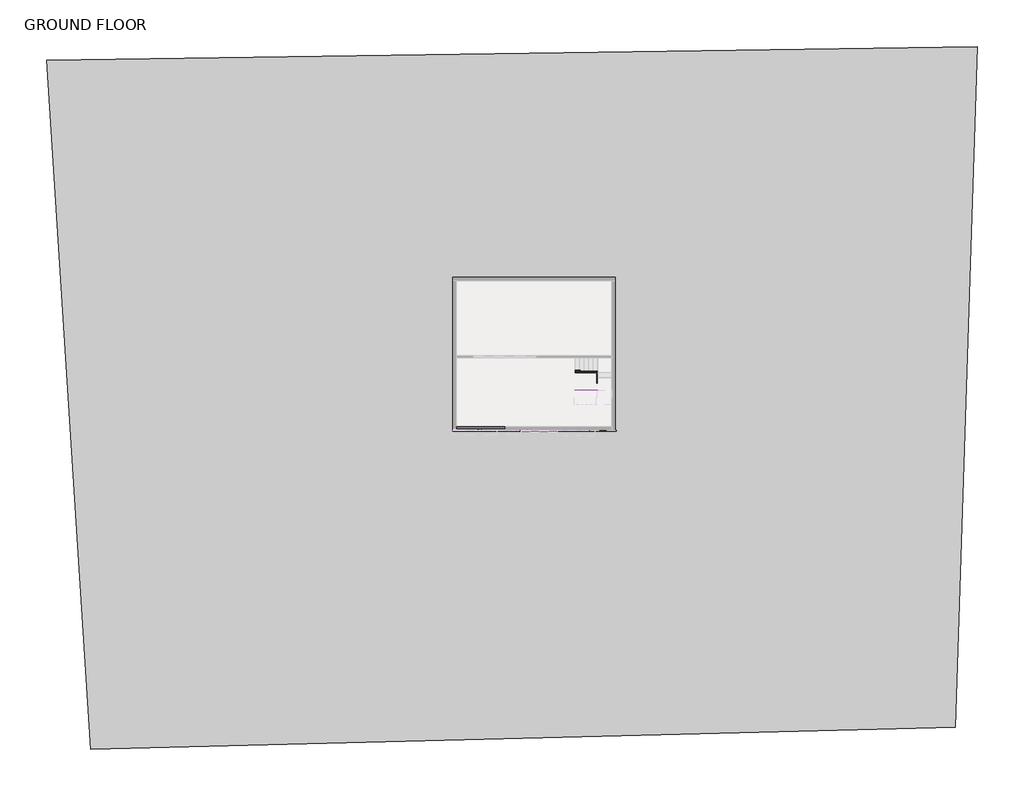
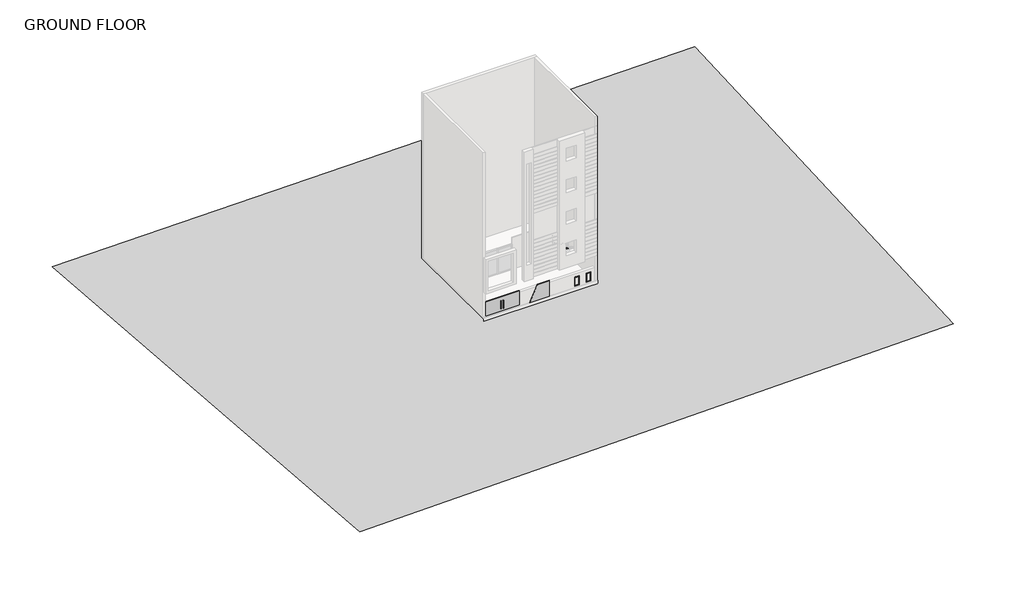
# One storey, part 3 of 3: 4 members, 3 proxies, 1 railing.
"""IFC4 building model written with IfcOpenShell, lengths in millimetres."""

from ifc_helpers import new_model, si_unit, frame, origin, place, context, project, spatial, polyline, circle_curve, ellipse_curve, outline, extrude, triangles, transform, mapped, element, save
from ifc_brep_helpers import plane_surface, cylinder_surface, advanced_brep
from components import generic_models_1_generic_models_1_bb1f4732, generic_models_2_generic_models_2_568ed07e

model = new_model("IFC4")

# Units and contexts
model_context = context("Model", 3, world=origin())
ifc_project = project(units=[si_unit("LENGTHUNIT", "METRE", prefix="MILLI")], contexts=[model_context])

# Site, building, storey
site = spatial("IfcSite", under=ifc_project)
building = spatial("IfcBuilding", under=site)
storey = spatial("IfcBuildingStorey", under=building, Name="GROUND FLOOR", Elevation=304.8)

# Proxies
placement = place(None, origin())
element("IfcBuildingElementProxy", 1, Name="Building Element Proxy", at=placement, inside=storey, context=model_context, shape_type="Tessellation", body=[
    triangles([(-29534.7437439, -19838.4774536, 0.0), (25460.3133728, -18431.1226593, 0.0), (-32349.4533325, 24006.0091187, 0.0), (26867.6670044, 24872.0725342, 0.0)], [[3, 1, 2], [2, 4, 3]], closed=False),
])
generic_models_1_generic_models_1_shape = generic_models_1_generic_models_1_bb1f4732(model_context)
element("IfcBuildingElementProxy", 2, Name="Generic Models 1 : Generic Models 1", ObjectType="Generic Models 1 : Generic Models 1", at=placement, inside=storey, context=model_context, shape_type="MappedRepresentation", body=[
    mapped(generic_models_1_generic_models_1_shape, transform((0.0, 0.0, 0.0), x_axis=(1.0, 0.0, 0.0), y_axis=(0.0, 1.0, 0.0), z_axis=(0.0, 0.0, 1.0))),
])
generic_models_2_generic_models_2_shape = generic_models_2_generic_models_2_568ed07e(model_context)
element("IfcBuildingElementProxy", 3, Name="Generic Models 2 : Generic Models 2", ObjectType="Generic Models 2 : Generic Models 2", at=placement, inside=storey, context=model_context, shape_type="MappedRepresentation", body=[
    mapped(generic_models_2_generic_models_2_shape, transform((0.0, 0.0, 0.0), x_axis=(1.0, 0.0, 0.0), y_axis=(0.0, 1.0, 0.0), z_axis=(0.0, 0.0, 1.0))),
])

# Members
element("IfcMember", 4, ObjectType="Stringer - 2\" Width", at=placement, inside=storey, context=model_context, shape_type="SweptSolid", body=[
    extrude(outline(polyline([(514.3152483, 1298.3430349), (304.8, 1298.3430349), (304.8, 1545.0209868), (969.1571187, 2695.3430349), (1321.1387777, 2695.3430349), (514.3152483, 1298.3430349)])), frame((0.0, 5080.6555142, 0.0), z_axis=(0.0, 1.0, 0.0), x_axis=(0.0, 0.0, 1.0)), (0.0, 0.0, 1.0), 50.8),
])
element("IfcMember", 5, ObjectType="Stringer - 2\" Width", at=placement, inside=storey, context=model_context, shape_type="SweptSolid", body=[
    extrude(outline(polyline([(514.3152483, 1298.3430349), (304.8, 1298.3430349), (304.8, 1545.0209868), (969.1571187, 2695.3430349), (1321.1387777, 2695.3430349), (514.3152483, 1298.3430349)])), frame((0.0, 4115.4555142, 0.0), z_axis=(0.0, 1.0, 0.0), x_axis=(0.0, 0.0, 1.0)), (0.0, 0.0, 1.0), 50.8),
])
element("IfcMember", 6, ObjectType="Stringer - 2\" Width", at=placement, inside=storey, context=model_context, shape_type="SweptSolid", body=[
    extrude(outline(polyline([(4115.4555142, 1482.5034836), (4115.4555142, 1130.5218246), (3048.6555142, 1746.6416107), (3048.6555142, 2098.6232697), (4115.4555142, 1482.5034836)])), frame((2644.5430349, 0.0, 0.0), z_axis=(1.0, 0.0, 0.0), x_axis=(0.0, 1.0, 0.0)), (0.0, 0.0, 1.0), 50.8),
])
element("IfcMember", 7, ObjectType="Stringer - 2\" Width", at=placement, inside=storey, context=model_context, shape_type="SweptSolid", body=[
    extrude(outline(polyline([(1908.0063166, 2695.3430349), (2259.9879755, 2695.3430349), (3096.1505424, 1247.5430349), (2744.1688834, 1247.5430349), (1908.0063166, 2695.3430349)])), frame((0.0, 2997.8555142, 0.0), z_axis=(0.0, 1.0, 0.0), x_axis=(0.0, 0.0, 1.0)), (0.0, 0.0, 1.0), 50.8),
])

# Railing
element("IfcRailing", 8, ObjectType="Guardrail - Pipe", at=placement, inside=storey, context=model_context, shape_type="AdvancedBrep", body=[
    advanced_brep(
    [(1298.3430349, 4248.8055142, 1358.5658522), (1298.3430349, 4286.9055142, 1358.5658522), (2695.3430349, 4248.8055142, 2165.3893816), (2695.3430349, 4286.9055142, 2165.3893816)],
    [
        (0, 1, ellipse_curve(frame((1298.3430349, 4267.8555142, 1358.5658522), z_axis=(-1.0, 0.0, 0.0), x_axis=(0.0, 0.0, -1.0)), 21.9988537, 19.05)),
        (1, 0, ellipse_curve(frame((1298.3430349, 4267.8555142, 1358.5658522), z_axis=(-1.0, 0.0, 0.0), x_axis=(0.0, 0.0, -1.0)), 21.9988537, 19.05)),
        (2, 3, ellipse_curve(frame((2695.3430349, 4267.8555142, 2165.3893816), z_axis=(1.0, 0.0, 0.0), x_axis=(0.0, 0.0, -1.0)), 21.9988537, 19.05)),
        (3, 2, ellipse_curve(frame((2695.3430349, 4267.8555142, 2165.3893816), z_axis=(1.0, 0.0, 0.0), x_axis=(0.0, 0.0, -1.0)), 21.9988537, 19.05)),
        (0, 2),
        (3, 1),
    ],
    [
        plane_surface(frame((1298.3430349, 4267.8555142, 1380.5647059), z_axis=(-1.0, 0.0, 0.0), x_axis=(0.0, 1.0, 0.0))),
        plane_surface(frame((2695.3430349, 4267.8555142, 2187.3882353), z_axis=(1.0, 0.0, 0.0), x_axis=(0.0, 1.0, 0.0))),
        cylinder_surface(frame((1307.8703836, 4267.8555142, 1364.0682781), z_axis=(-0.8659542116993035, 0.0, -0.5001232880402972), x_axis=(0.0, 1.0, 0.0)), 19.05),
    ],
    [
        (0, [[1, 2]]),
        (1, [[3, 4]]),
        (2, [[-1, 5, -4, 6]]),
        (2, [[-2, -6, -3, -5]]),
    ],
),
    advanced_brep(
    [(1298.3430349, 4172.6055142, 1510.9658522), (1298.3430349, 4210.7055142, 1510.9658522), (2695.3430349, 4172.6055142, 2317.7893816), (2695.3430349, 4210.7055142, 2317.7893816)],
    [
        (0, 1, ellipse_curve(frame((1298.3430349, 4191.6555142, 1510.9658522), z_axis=(-1.0, 0.0, 0.0), x_axis=(0.0, 0.0, -1.0)), 21.9988537, 19.05)),
        (1, 0, ellipse_curve(frame((1298.3430349, 4191.6555142, 1510.9658522), z_axis=(-1.0, 0.0, 0.0), x_axis=(0.0, 0.0, -1.0)), 21.9988537, 19.05)),
        (2, 3, ellipse_curve(frame((2695.3430349, 4191.6555142, 2317.7893816), z_axis=(1.0, 0.0, 0.0), x_axis=(0.0, 0.0, -1.0)), 21.9988537, 19.05)),
        (3, 2, ellipse_curve(frame((2695.3430349, 4191.6555142, 2317.7893816), z_axis=(1.0, 0.0, 0.0), x_axis=(0.0, 0.0, -1.0)), 21.9988537, 19.05)),
        (0, 2),
        (3, 1),
    ],
    [
        plane_surface(frame((1298.3430349, 4191.6555142, 1532.9647059), z_axis=(-1.0, 0.0, 0.0), x_axis=(0.0, 1.0, 0.0))),
        plane_surface(frame((2695.3430349, 4191.6555142, 2339.7882353), z_axis=(1.0, 0.0, 0.0), x_axis=(0.0, 1.0, 0.0))),
        cylinder_surface(frame((1307.8703836, 4191.6555142, 1516.4682781), z_axis=(-0.8659542116993035, 0.0, -0.5001232880402972), x_axis=(0.0, 1.0, 0.0)), 19.05),
    ],
    [
        (0, [[1, 2]]),
        (1, [[3, 4]]),
        (2, [[-1, 5, -4, 6]]),
        (2, [[-2, -6, -3, -5]]),
    ],
),
    advanced_brep(
    [(1298.3430349, 4204.3555142, 1365.8988034), (1298.3430349, 4178.9555142, 1365.8988034), (2695.3430349, 4204.3555142, 2172.7223328), (2695.3430349, 4178.9555142, 2172.7223328)],
    [
        (0, 1, ellipse_curve(frame((1298.3430349, 4191.6555142, 1365.8988034), z_axis=(-1.0, 0.0, 0.0), x_axis=(0.0, 0.0, -1.0)), 14.6659025, 12.7)),
        (1, 0, ellipse_curve(frame((1298.3430349, 4191.6555142, 1365.8988034), z_axis=(-1.0, 0.0, 0.0), x_axis=(0.0, 0.0, -1.0)), 14.6659025, 12.7)),
        (2, 3, ellipse_curve(frame((2695.3430349, 4191.6555142, 2172.7223328), z_axis=(1.0, 0.0, 0.0), x_axis=(0.0, 0.0, -1.0)), 14.6659025, 12.7)),
        (3, 2, ellipse_curve(frame((2695.3430349, 4191.6555142, 2172.7223328), z_axis=(1.0, 0.0, 0.0), x_axis=(0.0, 0.0, -1.0)), 14.6659025, 12.7)),
        (0, 2),
        (3, 1),
    ],
    [
        plane_surface(frame((1298.3430349, 4191.6555142, 1380.5647059), z_axis=(-1.0, 0.0, 0.0), x_axis=(0.0, 1.0, 0.0))),
        plane_surface(frame((2695.3430349, 4191.6555142, 2187.3882353), z_axis=(1.0, 0.0, 0.0), x_axis=(0.0, 1.0, 0.0))),
        cylinder_surface(frame((1304.6946007, 4191.6555142, 1369.5670874), z_axis=(-0.8659542116993035, 0.0, -0.5001232880402972), x_axis=(0.0, -1.0, 0.0)), 12.7),
    ],
    [
        (0, [[1, 2]]),
        (1, [[3, 4]]),
        (2, [[-1, 5, -4, 6]]),
        (2, [[-2, -6, -3, -5]]),
    ],
),
    advanced_brep(
    [(1298.3430349, 4204.3555142, 1238.8988034), (1298.3430349, 4178.9555142, 1238.8988034), (2695.3430349, 4204.3555142, 2045.7223328), (2695.3430349, 4178.9555142, 2045.7223328)],
    [
        (0, 1, ellipse_curve(frame((1298.3430349, 4191.6555142, 1238.8988034), z_axis=(-1.0, 0.0, 0.0), x_axis=(0.0, 0.0, -1.0)), 14.6659025, 12.7)),
        (1, 0, ellipse_curve(frame((1298.3430349, 4191.6555142, 1238.8988034), z_axis=(-1.0, 0.0, 0.0), x_axis=(0.0, 0.0, -1.0)), 14.6659025, 12.7)),
        (2, 3, ellipse_curve(frame((2695.3430349, 4191.6555142, 2045.7223328), z_axis=(1.0, 0.0, 0.0), x_axis=(0.0, 0.0, -1.0)), 14.6659025, 12.7)),
        (3, 2, ellipse_curve(frame((2695.3430349, 4191.6555142, 2045.7223328), z_axis=(1.0, 0.0, 0.0), x_axis=(0.0, 0.0, -1.0)), 14.6659025, 12.7)),
        (0, 2),
        (3, 1),
    ],
    [
        plane_surface(frame((1298.3430349, 4191.6555142, 1253.5647059), z_axis=(-1.0, 0.0, 0.0), x_axis=(0.0, 1.0, 0.0))),
        plane_surface(frame((2695.3430349, 4191.6555142, 2060.3882353), z_axis=(1.0, 0.0, 0.0), x_axis=(0.0, 1.0, 0.0))),
        cylinder_surface(frame((1304.6946007, 4191.6555142, 1242.5670874), z_axis=(-0.8659542116993035, 0.0, -0.5001232880402972), x_axis=(0.0, -1.0, 0.0)), 12.7),
    ],
    [
        (0, [[1, 2]]),
        (1, [[3, 4]]),
        (2, [[-1, 5, -4, 6]]),
        (2, [[-2, -6, -3, -5]]),
    ],
),
    advanced_brep(
    [(1298.3430349, 4204.3555142, 1111.8988034), (1298.3430349, 4178.9555142, 1111.8988034), (2695.3430349, 4204.3555142, 1918.7223328), (2695.3430349, 4178.9555142, 1918.7223328)],
    [
        (0, 1, ellipse_curve(frame((1298.3430349, 4191.6555142, 1111.8988034), z_axis=(-1.0, 0.0, 0.0), x_axis=(0.0, 0.0, -1.0)), 14.6659025, 12.7)),
        (1, 0, ellipse_curve(frame((1298.3430349, 4191.6555142, 1111.8988034), z_axis=(-1.0, 0.0, 0.0), x_axis=(0.0, 0.0, -1.0)), 14.6659025, 12.7)),
        (2, 3, ellipse_curve(frame((2695.3430349, 4191.6555142, 1918.7223328), z_axis=(1.0, 0.0, 0.0), x_axis=(0.0, 0.0, -1.0)), 14.6659025, 12.7)),
        (3, 2, ellipse_curve(frame((2695.3430349, 4191.6555142, 1918.7223328), z_axis=(1.0, 0.0, 0.0), x_axis=(0.0, 0.0, -1.0)), 14.6659025, 12.7)),
        (0, 2),
        (3, 1),
    ],
    [
        plane_surface(frame((1298.3430349, 4191.6555142, 1126.5647059), z_axis=(-1.0, 0.0, 0.0), x_axis=(0.0, 1.0, 0.0))),
        plane_surface(frame((2695.3430349, 4191.6555142, 1933.3882353), z_axis=(1.0, 0.0, 0.0), x_axis=(0.0, 1.0, 0.0))),
        cylinder_surface(frame((1304.6946007, 4191.6555142, 1115.5670874), z_axis=(-0.8659542116993035, 0.0, -0.5001232880402972), x_axis=(0.0, -1.0, 0.0)), 12.7),
    ],
    [
        (0, [[1, 2]]),
        (1, [[3, 4]]),
        (2, [[-1, 5, -4, 6]]),
        (2, [[-2, -6, -3, -5]]),
    ],
),
    advanced_brep(
    [(1298.3430349, 4204.3555142, 984.8988034), (1298.3430349, 4178.9555142, 984.8988034), (2695.3430349, 4204.3555142, 1791.7223328), (2695.3430349, 4178.9555142, 1791.7223328)],
    [
        (0, 1, ellipse_curve(frame((1298.3430349, 4191.6555142, 984.8988034), z_axis=(-1.0, 0.0, 0.0), x_axis=(0.0, 0.0, -1.0)), 14.6659025, 12.7)),
        (1, 0, ellipse_curve(frame((1298.3430349, 4191.6555142, 984.8988034), z_axis=(-1.0, 0.0, 0.0), x_axis=(0.0, 0.0, -1.0)), 14.6659025, 12.7)),
        (2, 3, ellipse_curve(frame((2695.3430349, 4191.6555142, 1791.7223328), z_axis=(1.0, 0.0, 0.0), x_axis=(0.0, 0.0, -1.0)), 14.6659025, 12.7)),
        (3, 2, ellipse_curve(frame((2695.3430349, 4191.6555142, 1791.7223328), z_axis=(1.0, 0.0, 0.0), x_axis=(0.0, 0.0, -1.0)), 14.6659025, 12.7)),
        (0, 2),
        (3, 1),
    ],
    [
        plane_surface(frame((1298.3430349, 4191.6555142, 999.5647059), z_axis=(-1.0, 0.0, 0.0), x_axis=(0.0, 1.0, 0.0))),
        plane_surface(frame((2695.3430349, 4191.6555142, 1806.3882353), z_axis=(1.0, 0.0, 0.0), x_axis=(0.0, 1.0, 0.0))),
        cylinder_surface(frame((1304.6946007, 4191.6555142, 988.5670874), z_axis=(-0.8659542116993035, 0.0, -0.5001232880402972), x_axis=(0.0, -1.0, 0.0)), 12.7),
    ],
    [
        (0, [[1, 2]]),
        (1, [[3, 4]]),
        (2, [[-1, 5, -4, 6]]),
        (2, [[-2, -6, -3, -5]]),
    ],
),
    advanced_brep(
    [(1298.3430349, 4204.3555142, 857.8988034), (1298.3430349, 4178.9555142, 857.8988034), (2695.3430349, 4204.3555142, 1664.7223328), (2695.3430349, 4178.9555142, 1664.7223328)],
    [
        (0, 1, ellipse_curve(frame((1298.3430349, 4191.6555142, 857.8988034), z_axis=(-1.0, 0.0, 0.0), x_axis=(0.0, 0.0, -1.0)), 14.6659025, 12.7)),
        (1, 0, ellipse_curve(frame((1298.3430349, 4191.6555142, 857.8988034), z_axis=(-1.0, 0.0, 0.0), x_axis=(0.0, 0.0, -1.0)), 14.6659025, 12.7)),
        (2, 3, ellipse_curve(frame((2695.3430349, 4191.6555142, 1664.7223328), z_axis=(1.0, 0.0, 0.0), x_axis=(0.0, 0.0, -1.0)), 14.6659025, 12.7)),
        (3, 2, ellipse_curve(frame((2695.3430349, 4191.6555142, 1664.7223328), z_axis=(1.0, 0.0, 0.0), x_axis=(0.0, 0.0, -1.0)), 14.6659025, 12.7)),
        (0, 2),
        (3, 1),
    ],
    [
        plane_surface(frame((1298.3430349, 4191.6555142, 872.5647059), z_axis=(-1.0, 0.0, 0.0), x_axis=(0.0, 1.0, 0.0))),
        plane_surface(frame((2695.3430349, 4191.6555142, 1679.3882353), z_axis=(1.0, 0.0, 0.0), x_axis=(0.0, 1.0, 0.0))),
        cylinder_surface(frame((1304.6946007, 4191.6555142, 861.5670874), z_axis=(-0.8659542116993035, 0.0, -0.5001232880402972), x_axis=(0.0, -1.0, 0.0)), 12.7),
    ],
    [
        (0, [[1, 2]]),
        (1, [[3, 4]]),
        (2, [[-1, 5, -4, 6]]),
        (2, [[-2, -6, -3, -5]]),
    ],
),
    advanced_brep(
    [(1298.3430349, 4204.3555142, 730.8988034), (1298.3430349, 4178.9555142, 730.8988034), (2695.3430349, 4204.3555142, 1537.7223328), (2695.3430349, 4178.9555142, 1537.7223328)],
    [
        (0, 1, ellipse_curve(frame((1298.3430349, 4191.6555142, 730.8988034), z_axis=(-1.0, 0.0, 0.0), x_axis=(0.0, 0.0, -1.0)), 14.6659025, 12.7)),
        (1, 0, ellipse_curve(frame((1298.3430349, 4191.6555142, 730.8988034), z_axis=(-1.0, 0.0, 0.0), x_axis=(0.0, 0.0, -1.0)), 14.6659025, 12.7)),
        (2, 3, ellipse_curve(frame((2695.3430349, 4191.6555142, 1537.7223328), z_axis=(1.0, 0.0, 0.0), x_axis=(0.0, 0.0, -1.0)), 14.6659025, 12.7)),
        (3, 2, ellipse_curve(frame((2695.3430349, 4191.6555142, 1537.7223328), z_axis=(1.0, 0.0, 0.0), x_axis=(0.0, 0.0, -1.0)), 14.6659025, 12.7)),
        (0, 2),
        (3, 1),
    ],
    [
        plane_surface(frame((1298.3430349, 4191.6555142, 745.5647059), z_axis=(-1.0, 0.0, 0.0), x_axis=(0.0, 1.0, 0.0))),
        plane_surface(frame((2695.3430349, 4191.6555142, 1552.3882353), z_axis=(1.0, 0.0, 0.0), x_axis=(0.0, 1.0, 0.0))),
        cylinder_surface(frame((1304.6946007, 4191.6555142, 734.5670874), z_axis=(-0.8659542116993035, 0.0, -0.5001232880402972), x_axis=(0.0, -1.0, 0.0)), 12.7),
    ],
    [
        (0, [[1, 2]]),
        (1, [[3, 4]]),
        (2, [[-1, 5, -4, 6]]),
        (2, [[-2, -6, -3, -5]]),
    ],
),
    advanced_brep(
    [(1298.3430349, 4204.3555142, 603.8988034), (1298.3430349, 4178.9555142, 603.8988034), (2695.3430349, 4204.3555142, 1410.7223328), (2695.3430349, 4178.9555142, 1410.7223328)],
    [
        (0, 1, ellipse_curve(frame((1298.3430349, 4191.6555142, 603.8988034), z_axis=(-1.0, 0.0, 0.0), x_axis=(0.0, 0.0, -1.0)), 14.6659025, 12.7)),
        (1, 0, ellipse_curve(frame((1298.3430349, 4191.6555142, 603.8988034), z_axis=(-1.0, 0.0, 0.0), x_axis=(0.0, 0.0, -1.0)), 14.6659025, 12.7)),
        (2, 3, ellipse_curve(frame((2695.3430349, 4191.6555142, 1410.7223328), z_axis=(1.0, 0.0, 0.0), x_axis=(0.0, 0.0, -1.0)), 14.6659025, 12.7)),
        (3, 2, ellipse_curve(frame((2695.3430349, 4191.6555142, 1410.7223328), z_axis=(1.0, 0.0, 0.0), x_axis=(0.0, 0.0, -1.0)), 14.6659025, 12.7)),
        (0, 2),
        (3, 1),
    ],
    [
        plane_surface(frame((1298.3430349, 4191.6555142, 618.5647059), z_axis=(-1.0, 0.0, 0.0), x_axis=(0.0, 1.0, 0.0))),
        plane_surface(frame((2695.3430349, 4191.6555142, 1425.3882353), z_axis=(1.0, 0.0, 0.0), x_axis=(0.0, 1.0, 0.0))),
        cylinder_surface(frame((1304.6946007, 4191.6555142, 607.5670874), z_axis=(-0.8659542116993035, 0.0, -0.5001232880402972), x_axis=(0.0, -1.0, 0.0)), 12.7),
    ],
    [
        (0, [[1, 2]]),
        (1, [[3, 4]]),
        (2, [[-1, 5, -4, 6]]),
        (2, [[-2, -6, -3, -5]]),
    ],
),
    advanced_brep(
    [(2517.5430349, 4178.9555142, 2193.1038969), (2517.5430349, 4178.9555142, 1111.6235294), (2517.5430349, 4204.3555142, 1111.6235294), (2517.5430349, 4204.3555142, 2193.1038969)],
    [
        (0, 1),
        (1, 2, circle_curve(frame((2517.5430349, 4191.6555142, 1111.6235294), z_axis=(0.0, 0.0, 1.0), x_axis=(0.0, 1.0, 0.0)), 12.7)),
        (2, 3),
        (3, 0, ellipse_curve(frame((2517.5430349, 4191.6555142, 2193.1038969), z_axis=(0.5001232880402952, 0.0, -0.8659542116993046), x_axis=(0.8659542116993046, 0.0, 0.5001232880402949)), 14.6659025, 12.7)),
        (0, 3, ellipse_curve(frame((2517.5430349, 4191.6555142, 2193.1038969), z_axis=(0.5001232880402952, 0.0, -0.8659542116993046), x_axis=(0.8659542116993046, 0.0, 0.5001232880402949)), 14.6659025, 12.7)),
        (2, 1, circle_curve(frame((2517.5430349, 4191.6555142, 1111.6235294), z_axis=(0.0, 0.0, 1.0), x_axis=(0.0, 1.0, 0.0)), 12.7)),
    ],
    [
        cylinder_surface(frame((2517.5430349, 4191.6555142, 883.0235294), z_axis=(0.0, 0.0, 1.0), x_axis=(0.0, 1.0, 0.0)), 12.7),
        plane_surface(frame((2542.9430349, 4217.0555142, 2207.7734156), z_axis=(-0.5001232880402952, 0.0, 0.8659542116993046), x_axis=(0.0, -1.0, 0.0))),
        plane_surface(frame((2492.1430349, 4217.0555142, 1111.6235294), z_axis=(0.0, 0.0, -1.0), x_axis=(0.0, -1.0, 0.0))),
    ],
    [
        (0, [[1, 2, 3, 4]]),
        (0, [[-1, 5, -3, 6]]),
        (1, [[-4, -5]]),
        (2, [[-2, -6]]),
    ],
),
    advanced_brep(
    [(2682.6430349, 4178.9555142, 2288.4557686), (2682.6430349, 4178.9555142, 1111.6235294), (2682.6430349, 4204.3555142, 1111.6235294), (2682.6430349, 4204.3555142, 2288.4557686)],
    [
        (0, 1),
        (1, 2, circle_curve(frame((2682.6430349, 4191.6555142, 1111.6235294), z_axis=(0.0, 0.0, 1.0), x_axis=(0.0, 1.0, 0.0)), 12.7)),
        (2, 3),
        (3, 0, ellipse_curve(frame((2682.6430349, 4191.6555142, 2288.4557686), z_axis=(0.5001232880402952, 0.0, -0.8659542116993046), x_axis=(0.8659542116993046, 0.0, 0.5001232880402949)), 14.6659025, 12.7)),
        (0, 3, ellipse_curve(frame((2682.6430349, 4191.6555142, 2288.4557686), z_axis=(0.5001232880402952, 0.0, -0.8659542116993046), x_axis=(0.8659542116993046, 0.0, 0.5001232880402949)), 14.6659025, 12.7)),
        (2, 1, circle_curve(frame((2682.6430349, 4191.6555142, 1111.6235294), z_axis=(0.0, 0.0, 1.0), x_axis=(0.0, 1.0, 0.0)), 12.7)),
    ],
    [
        cylinder_surface(frame((2682.6430349, 4191.6555142, 883.0235294), z_axis=(0.0, 0.0, 1.0), x_axis=(0.0, 1.0, 0.0)), 12.7),
        plane_surface(frame((2708.0430349, 4217.0555142, 2303.1252873), z_axis=(-0.5001232880402952, 0.0, 0.8659542116993046), x_axis=(0.0, -1.0, 0.0))),
        plane_surface(frame((2657.2430349, 4217.0555142, 1111.6235294), z_axis=(0.0, 0.0, -1.0), x_axis=(0.0, -1.0, 0.0))),
    ],
    [
        (0, [[1, 2, 3, 4]]),
        (0, [[-1, 5, -3, 6]]),
        (1, [[-4, -5]]),
        (2, [[-2, -6]]),
    ],
),
    advanced_brep(
    [(1311.0430349, 4178.9555142, 1496.3017579), (1311.0430349, 4178.9555142, 466.1647059), (1311.0430349, 4204.3555142, 466.1647059), (1311.0430349, 4204.3555142, 1496.3017579)],
    [
        (0, 1),
        (1, 2, circle_curve(frame((1311.0430349, 4191.6555142, 466.1647059), z_axis=(0.0, 0.0, 1.0), x_axis=(0.0, 1.0, 0.0)), 12.7)),
        (2, 3),
        (3, 0, ellipse_curve(frame((1311.0430349, 4191.6555142, 1496.3017579), z_axis=(0.5001232880402935, 0.0, -0.8659542116993056), x_axis=(0.8659542116993056, 0.0, 0.500123288040293)), 14.6659025, 12.7)),
        (0, 3, ellipse_curve(frame((1311.0430349, 4191.6555142, 1496.3017579), z_axis=(0.5001232880402935, 0.0, -0.8659542116993056), x_axis=(0.8659542116993056, 0.0, 0.500123288040293)), 14.6659025, 12.7)),
        (2, 1, circle_curve(frame((1311.0430349, 4191.6555142, 466.1647059), z_axis=(0.0, 0.0, 1.0), x_axis=(0.0, 1.0, 0.0)), 12.7)),
    ],
    [
        cylinder_surface(frame((1311.0430349, 4191.6555142, 237.5647059), z_axis=(0.0, 0.0, 1.0), x_axis=(0.0, 1.0, 0.0)), 12.7),
        plane_surface(frame((1336.4430349, 4217.0555142, 1510.9712766), z_axis=(-0.5001232880402935, 0.0, 0.8659542116993056), x_axis=(0.0, -1.0, 0.0))),
        plane_surface(frame((1285.6430349, 4217.0555142, 466.1647059), z_axis=(0.0, 0.0, -1.0), x_axis=(0.0, -1.0, 0.0))),
    ],
    [
        (0, [[1, 2, 3, 4]]),
        (0, [[-1, 5, -3, 6]]),
        (1, [[-4, -5]]),
        (2, [[-2, -6]]),
    ],
),
])

save(model, "model.ifc")

# Revit data of these elements
# Type "Guardrail - Pipe"
#   Assembly Code = "C2010400"
#   built-in parameter 1008612 = 0.0416667 (stored number, unit not read)
#   built-in parameter 1008611 = 0.0833333 (stored number, unit not read)
#   built-in parameter 1008609 = 4 (stored number, unit not read)
#   built-in parameter 1008604 = 0.166667 (stored number, unit not read)
#   built-in parameter 1008603 = 0.166667 (stored number, unit not read)
#   Railing Height = 3' - 6"
#   built-in parameter 1008630 = 2
#   built-in parameter 1008610 = 1
#   built-in parameter 1008605 = 1
#   built-in parameter 1008618 = Baluster - Round : 1"
# Element 1 (IfcBuildingElementProxy)
#   Material = 1 grass
#   Phase Created = New Construction
# Element 2 (IfcBuildingElementProxy, "Generic Models 1 : Generic Models 1")
#   Phase Created = New Construction
#   Materials on its faces: "1 wood", "1 wall brown"
# Element 3 (IfcBuildingElementProxy, "Generic Models 2 : Generic Models 2")
#   Phase Created = New Construction
#   Materials on its faces: "1 wall brown", "1 wall white"
# Elements 4, 5, 6, 7 (IfcMember, "Stringer - 2\" Width")
#   Phase Created = New Construction
# Element 8 (IfcRailing, "Guardrail - Pipe")
#   Phase Created = New Construction
# Materials
#   "1 grass": class "Generic", colour RGB 43 79 37, transparency 0, Cost = 0
#   "1 wood": class "Generic", colour RGB 120 120 120, transparency 0, Cost = 0
#   "1 wall brown": class "Generic", colour RGB 61 46 37, transparency 0, Cost = 0
#   "1 wall white": class "Generic", colour RGB 244 245 241, transparency 0, Cost = 0
